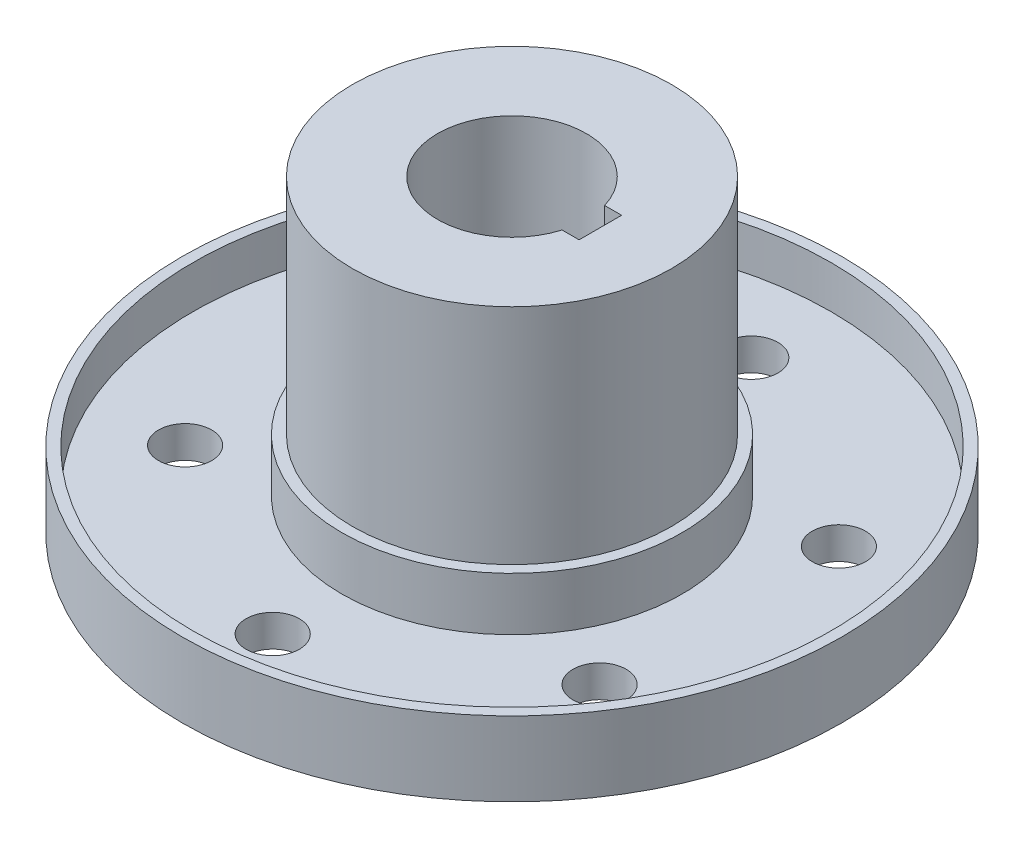
ISO-10303-21;
HEADER;
FILE_DESCRIPTION(('STEP AP214'),'2;1');
FILE_NAME('part.step','',(''),(''),'','','');
FILE_SCHEMA(('AUTOMOTIVE_DESIGN { 1 0 10303 214 1 1 1 1 }'));
ENDSEC;
DATA;
#1=APPLICATION_CONTEXT('core data for automotive mechanical design processes');
#2=APPLICATION_PROTOCOL_DEFINITION('international standard','automotive_design',2000,#1);
#3=PRODUCT_CONTEXT('',#1,'mechanical');
#4=PRODUCT('Part','Part','',(#3));
#5=PRODUCT_RELATED_PRODUCT_CATEGORY('part','',(#4));
#6=PRODUCT_DEFINITION_FORMATION('','',#4);
#7=PRODUCT_DEFINITION_CONTEXT('part definition',#1,'design');
#8=PRODUCT_DEFINITION('design','',#6,#7);
#9=PRODUCT_DEFINITION_SHAPE('','',#8);
#10=(LENGTH_UNIT() NAMED_UNIT(*) SI_UNIT(.MILLI.,.METRE.));
#11=(NAMED_UNIT(*) PLANE_ANGLE_UNIT() SI_UNIT($,.RADIAN.));
#12=(NAMED_UNIT(*) SI_UNIT($,.STERADIAN.) SOLID_ANGLE_UNIT());
#13=UNCERTAINTY_MEASURE_WITH_UNIT(LENGTH_MEASURE(1.E-05),#10,'distance_accuracy_value','');
#14=(GEOMETRIC_REPRESENTATION_CONTEXT(3) GLOBAL_UNCERTAINTY_ASSIGNED_CONTEXT((#13)) GLOBAL_UNIT_ASSIGNED_CONTEXT((#10,
#11,#12)) REPRESENTATION_CONTEXT('',''));
#15=CARTESIAN_POINT('',(0.,0.,0.));
#16=DIRECTION('',(0.,0.,1.));
#17=DIRECTION('',(1.,0.,0.));
#18=AXIS2_PLACEMENT_3D('',#15,#16,#17);
#19=CARTESIAN_POINT('',(41.5410196624969,2.99999999999998,-10.));
#20=DIRECTION('',(1.,0.,0.));
#21=DIRECTION('',(0.,0.,-1.));
#22=AXIS2_PLACEMENT_3D('',#19,#20,#21);
#23=PLANE('',#22);
#24=DIRECTION('',(0.,0.,-1.));
#25=VECTOR('',#24,1.);
#26=CARTESIAN_POINT('',(41.5410196624969,50.,-10.));
#27=LINE('',#26,#25);
#28=CARTESIAN_POINT('',(41.5410196624969,50.,9.99999999999999));
#29=VERTEX_POINT('',#28);
#30=CARTESIAN_POINT('',(41.5410196624969,50.,-10.));
#31=VERTEX_POINT('',#30);
#32=EDGE_CURVE('E52',#29,#31,#27,.T.);
#33=ORIENTED_EDGE('',*,*,#32,.F.);
#34=DIRECTION('',(0.,1.,0.));
#35=VECTOR('',#34,1.);
#36=CARTESIAN_POINT('',(41.5410196624969,2.99999999999998,9.99999999999999));
#37=LINE('',#36,#35);
#38=CARTESIAN_POINT('',(41.5410196624969,145.,9.99999999999999));
#39=VERTEX_POINT('',#38);
#40=EDGE_CURVE('E98',#29,#39,#37,.T.);
#41=ORIENTED_EDGE('',*,*,#40,.T.);
#42=DIRECTION('',(0.,0.,-1.));
#43=VECTOR('',#42,1.);
#44=CARTESIAN_POINT('',(41.5410196624969,145.,-10.));
#45=LINE('',#44,#43);
#46=CARTESIAN_POINT('',(41.5410196624969,145.,-10.));
#47=VERTEX_POINT('',#46);
#48=EDGE_CURVE('E372',#39,#47,#45,.T.);
#49=ORIENTED_EDGE('',*,*,#48,.T.);
#50=DIRECTION('',(0.,1.,0.));
#51=VECTOR('',#50,1.);
#52=CARTESIAN_POINT('',(41.5410196624969,2.99999999999998,-10.));
#53=LINE('',#52,#51);
#54=EDGE_CURVE('E58',#31,#47,#53,.T.);
#55=ORIENTED_EDGE('',*,*,#54,.F.);
#56=EDGE_LOOP('',(#33,#41,#49,#55));
#57=FACE_BOUND('',#56,.T.);
#58=ADVANCED_FACE('F39',(#57),#23,.F.);
#59=CARTESIAN_POINT('',(41.5410196624969,2.99999999999998,9.99999999999999));
#60=DIRECTION('',(0.,0.,1.));
#61=DIRECTION('',(1.,0.,0.));
#62=AXIS2_PLACEMENT_3D('',#59,#60,#61);
#63=PLANE('',#62);
#64=DIRECTION('',(1.,0.,0.));
#65=VECTOR('',#64,1.);
#66=CARTESIAN_POINT('',(41.5410196624969,50.,9.99999999999999));
#67=LINE('',#66,#65);
#68=CARTESIAN_POINT('',(33.5410196624969,50.,9.99999999999998));
#69=VERTEX_POINT('',#68);
#70=EDGE_CURVE('E88',#69,#29,#67,.T.);
#71=ORIENTED_EDGE('',*,*,#70,.F.);
#72=DIRECTION('',(0.,1.,0.));
#73=VECTOR('',#72,1.);
#74=CARTESIAN_POINT('',(33.5410196624969,2.99999999999998,9.99999999999998));
#75=LINE('',#74,#73);
#76=CARTESIAN_POINT('',(33.5410196624969,145.,9.99999999999998));
#77=VERTEX_POINT('',#76);
#78=EDGE_CURVE('E90',#69,#77,#75,.T.);
#79=ORIENTED_EDGE('',*,*,#78,.T.);
#80=DIRECTION('',(1.,0.,0.));
#81=VECTOR('',#80,1.);
#82=CARTESIAN_POINT('',(41.5410196624969,145.,9.99999999999999));
#83=LINE('',#82,#81);
#84=EDGE_CURVE('E96',#77,#39,#83,.T.);
#85=ORIENTED_EDGE('',*,*,#84,.T.);
#86=ORIENTED_EDGE('',*,*,#40,.F.);
#87=EDGE_LOOP('',(#71,#79,#85,#86));
#88=FACE_BOUND('',#87,.T.);
#89=ADVANCED_FACE('F185',(#88),#63,.F.);
#90=CARTESIAN_POINT('',(0.,2.99999999999998,0.));
#91=DIRECTION('',(0.,1.,0.));
#92=DIRECTION('',(0.,0.,1.));
#93=AXIS2_PLACEMENT_3D('',#90,#91,#92);
#94=CYLINDRICAL_SURFACE('',#93,35.);
#95=CARTESIAN_POINT('',(0.,50.,0.));
#96=DIRECTION('',(0.,-1.,0.));
#97=DIRECTION('',(0.,0.,-1.));
#98=AXIS2_PLACEMENT_3D('',#95,#96,#97);
#99=CIRCLE('',#98,35.);
#100=CARTESIAN_POINT('',(33.5410196624969,50.,-10.));
#101=VERTEX_POINT('',#100);
#102=EDGE_CURVE('E79',#101,#69,#99,.F.);
#103=ORIENTED_EDGE('',*,*,#102,.F.);
#104=DIRECTION('',(0.,1.,0.));
#105=VECTOR('',#104,1.);
#106=CARTESIAN_POINT('',(33.5410196624969,2.99999999999998,-10.));
#107=LINE('',#106,#105);
#108=CARTESIAN_POINT('',(33.5410196624969,145.,-10.));
#109=VERTEX_POINT('',#108);
#110=EDGE_CURVE('E86',#101,#109,#107,.T.);
#111=ORIENTED_EDGE('',*,*,#110,.T.);
#112=CARTESIAN_POINT('',(0.,145.,0.));
#113=DIRECTION('',(0.,1.,0.));
#114=DIRECTION('',(0.,0.,1.));
#115=AXIS2_PLACEMENT_3D('',#112,#113,#114);
#116=CIRCLE('',#115,35.);
#117=EDGE_CURVE('E380',#109,#77,#116,.T.);
#118=ORIENTED_EDGE('',*,*,#117,.T.);
#119=ORIENTED_EDGE('',*,*,#78,.F.);
#120=EDGE_LOOP('',(#103,#111,#118,#119));
#121=FACE_BOUND('',#120,.T.);
#122=ADVANCED_FACE('F81',(#121),#94,.F.);
#123=CARTESIAN_POINT('',(41.5410196624969,2.99999999999998,-10.));
#124=DIRECTION('',(0.,0.,-1.));
#125=DIRECTION('',(-1.,0.,0.));
#126=AXIS2_PLACEMENT_3D('',#123,#124,#125);
#127=PLANE('',#126);
#128=DIRECTION('',(-1.,0.,0.));
#129=VECTOR('',#128,1.);
#130=CARTESIAN_POINT('',(41.5410196624969,50.,-10.));
#131=LINE('',#130,#129);
#132=EDGE_CURVE('E11',#31,#101,#131,.T.);
#133=ORIENTED_EDGE('',*,*,#132,.F.);
#134=ORIENTED_EDGE('',*,*,#54,.T.);
#135=DIRECTION('',(-1.,0.,0.));
#136=VECTOR('',#135,1.);
#137=CARTESIAN_POINT('',(41.5410196624969,145.,-10.));
#138=LINE('',#137,#136);
#139=EDGE_CURVE('E92',#47,#109,#138,.T.);
#140=ORIENTED_EDGE('',*,*,#139,.T.);
#141=ORIENTED_EDGE('',*,*,#110,.F.);
#142=EDGE_LOOP('',(#133,#134,#140,#141));
#143=FACE_BOUND('',#142,.T.);
#144=ADVANCED_FACE('F91',(#143),#127,.F.);
#145=CARTESIAN_POINT('',(0.,35.,0.));
#146=DIRECTION('',(0.,1.,0.));
#147=DIRECTION('',(0.,0.,1.));
#148=AXIS2_PLACEMENT_3D('',#145,#146,#147);
#149=PLANE('',#148);
#150=CARTESIAN_POINT('',(0.,35.,0.));
#151=DIRECTION('',(0.,1.,0.));
#152=DIRECTION('',(0.,0.,1.));
#153=AXIS2_PLACEMENT_3D('',#150,#151,#152);
#154=CIRCLE('',#153,155.);
#155=CARTESIAN_POINT('',(0.,35.,155.));
#156=VERTEX_POINT('',#155);
#157=EDGE_CURVE('E152',#156,#156,#154,.T.);
#158=ORIENTED_EDGE('',*,*,#157,.T.);
#159=EDGE_LOOP('',(#158));
#160=FACE_BOUND('',#159,.T.);
#161=CARTESIAN_POINT('',(0.,35.,0.));
#162=DIRECTION('',(0.,1.,0.));
#163=DIRECTION('',(0.,0.,1.));
#164=AXIS2_PLACEMENT_3D('',#161,#162,#163);
#165=CIRCLE('',#164,150.);
#166=CARTESIAN_POINT('',(0.,35.,150.));
#167=VERTEX_POINT('',#166);
#168=EDGE_CURVE('E148',#167,#167,#165,.T.);
#169=ORIENTED_EDGE('',*,*,#168,.F.);
#170=EDGE_LOOP('',(#169));
#171=FACE_BOUND('',#170,.T.);
#172=ADVANCED_FACE('F169',(#160,#171),#149,.T.);
#173=CARTESIAN_POINT('',(0.,0.,0.));
#174=DIRECTION('',(0.,1.,0.));
#175=DIRECTION('',(0.,0.,1.));
#176=AXIS2_PLACEMENT_3D('',#173,#174,#175);
#177=PLANE('',#176);
#178=CARTESIAN_POINT('',(0.,0.,0.));
#179=DIRECTION('',(0.,-1.,0.));
#180=DIRECTION('',(0.,0.,-1.));
#181=AXIS2_PLACEMENT_3D('',#178,#179,#180);
#182=CIRCLE('',#181,60.);
#183=CARTESIAN_POINT('',(0.,0.,-60.));
#184=VERTEX_POINT('',#183);
#185=EDGE_CURVE('E368',#184,#184,#182,.T.);
#186=ORIENTED_EDGE('',*,*,#185,.F.);
#187=EDGE_LOOP('',(#186));
#188=FACE_BOUND('',#187,.T.);
#189=CARTESIAN_POINT('',(0.,0.,-112.5));
#190=DIRECTION('',(0.,1.,0.));
#191=DIRECTION('',(0.,0.,1.));
#192=AXIS2_PLACEMENT_3D('',#189,#190,#191);
#193=CIRCLE('',#192,12.5);
#194=CARTESIAN_POINT('',(0.,0.,-100.));
#195=VERTEX_POINT('',#194);
#196=EDGE_CURVE('E150',#195,#195,#193,.T.);
#197=ORIENTED_EDGE('',*,*,#196,.T.);
#198=EDGE_LOOP('',(#197));
#199=FACE_BOUND('',#198,.T.);
#200=CARTESIAN_POINT('',(-97.4278579257487,0.,-56.2500000000002));
#201=DIRECTION('',(0.,1.,0.));
#202=DIRECTION('',(0.,0.,1.));
#203=AXIS2_PLACEMENT_3D('',#200,#201,#202);
#204=CIRCLE('',#203,12.500000000001);
#205=CARTESIAN_POINT('',(-97.4278579257487,0.,-43.7499999999992));
#206=VERTEX_POINT('',#205);
#207=EDGE_CURVE('E144',#206,#206,#204,.T.);
#208=ORIENTED_EDGE('',*,*,#207,.T.);
#209=EDGE_LOOP('',(#208));
#210=FACE_BOUND('',#209,.T.);
#211=CARTESIAN_POINT('',(-97.4278579257485,0.,56.249999999999));
#212=DIRECTION('',(0.,1.,0.));
#213=DIRECTION('',(0.,0.,1.));
#214=AXIS2_PLACEMENT_3D('',#211,#212,#213);
#215=CIRCLE('',#214,12.5000000000009);
#216=CARTESIAN_POINT('',(-97.4278579257485,0.,68.75));
#217=VERTEX_POINT('',#216);
#218=EDGE_CURVE('E142',#217,#217,#215,.T.);
#219=ORIENTED_EDGE('',*,*,#218,.T.);
#220=EDGE_LOOP('',(#219));
#221=FACE_BOUND('',#220,.T.);
#222=CARTESIAN_POINT('',(2.51087448004034E-13,0.,112.499999999999));
#223=DIRECTION('',(0.,1.,0.));
#224=DIRECTION('',(0.,0.,1.));
#225=AXIS2_PLACEMENT_3D('',#222,#223,#224);
#226=CIRCLE('',#225,12.5000000000014);
#227=CARTESIAN_POINT('',(2.51087448004034E-13,0.,125.));
#228=VERTEX_POINT('',#227);
#229=EDGE_CURVE('E137',#228,#228,#226,.T.);
#230=ORIENTED_EDGE('',*,*,#229,.T.);
#231=EDGE_LOOP('',(#230));
#232=FACE_BOUND('',#231,.T.);
#233=CARTESIAN_POINT('',(97.4278579257489,0.,56.2499999999988));
#234=DIRECTION('',(0.,1.,0.));
#235=DIRECTION('',(0.,0.,1.));
#236=AXIS2_PLACEMENT_3D('',#233,#234,#235);
#237=CIRCLE('',#236,12.5000000000016);
#238=CARTESIAN_POINT('',(97.4278579257489,0.,68.7500000000004));
#239=VERTEX_POINT('',#238);
#240=EDGE_CURVE('E134',#239,#239,#237,.T.);
#241=ORIENTED_EDGE('',*,*,#240,.T.);
#242=EDGE_LOOP('',(#241));
#243=FACE_BOUND('',#242,.T.);
#244=CARTESIAN_POINT('',(97.4278579257488,0.,-56.2500000000005));
#245=DIRECTION('',(0.,1.,0.));
#246=DIRECTION('',(0.,0.,1.));
#247=AXIS2_PLACEMENT_3D('',#244,#245,#246);
#248=CIRCLE('',#247,12.500000000001);
#249=CARTESIAN_POINT('',(97.4278579257488,0.,-43.7499999999995));
#250=VERTEX_POINT('',#249);
#251=EDGE_CURVE('E117',#250,#250,#248,.T.);
#252=ORIENTED_EDGE('',*,*,#251,.T.);
#253=EDGE_LOOP('',(#252));
#254=FACE_BOUND('',#253,.T.);
#255=CARTESIAN_POINT('',(0.,0.,0.));
#256=DIRECTION('',(0.,1.,0.));
#257=DIRECTION('',(0.,0.,1.));
#258=AXIS2_PLACEMENT_3D('',#255,#256,#257);
#259=CIRCLE('',#258,155.);
#260=CARTESIAN_POINT('',(0.,0.,155.));
#261=VERTEX_POINT('',#260);
#262=EDGE_CURVE('E153',#261,#261,#259,.T.);
#263=ORIENTED_EDGE('',*,*,#262,.F.);
#264=EDGE_LOOP('',(#263));
#265=FACE_BOUND('',#264,.T.);
#266=ADVANCED_FACE('F171',(#188,#199,#210,#221,#232,#243,#254,#265),#177,.F.);
#267=CARTESIAN_POINT('',(0.,35.,0.));
#268=DIRECTION('',(0.,-1.,0.));
#269=DIRECTION('',(0.,0.,-1.));
#270=AXIS2_PLACEMENT_3D('',#267,#268,#269);
#271=CYLINDRICAL_SURFACE('',#270,155.);
#272=ORIENTED_EDGE('',*,*,#157,.F.);
#273=EDGE_LOOP('',(#272));
#274=FACE_BOUND('',#273,.T.);
#275=ORIENTED_EDGE('',*,*,#262,.T.);
#276=EDGE_LOOP('',(#275));
#277=FACE_BOUND('',#276,.T.);
#278=ADVANCED_FACE('F41',(#274,#277),#271,.T.);
#279=CARTESIAN_POINT('',(0.,35.,0.));
#280=DIRECTION('',(0.,-1.,0.));
#281=DIRECTION('',(0.,0.,-1.));
#282=AXIS2_PLACEMENT_3D('',#279,#280,#281);
#283=CYLINDRICAL_SURFACE('',#282,150.);
#284=CARTESIAN_POINT('',(0.,15.,0.));
#285=DIRECTION('',(0.,1.,0.));
#286=DIRECTION('',(0.,0.,1.));
#287=AXIS2_PLACEMENT_3D('',#284,#285,#286);
#288=CIRCLE('',#287,150.);
#289=CARTESIAN_POINT('',(0.,15.,150.));
#290=VERTEX_POINT('',#289);
#291=EDGE_CURVE('E108',#290,#290,#288,.T.);
#292=ORIENTED_EDGE('',*,*,#291,.F.);
#293=EDGE_LOOP('',(#292));
#294=FACE_BOUND('',#293,.T.);
#295=ORIENTED_EDGE('',*,*,#168,.T.);
#296=EDGE_LOOP('',(#295));
#297=FACE_BOUND('',#296,.T.);
#298=ADVANCED_FACE('F161',(#294,#297),#283,.F.);
#299=CARTESIAN_POINT('',(0.,15.,0.));
#300=DIRECTION('',(0.,1.,0.));
#301=DIRECTION('',(0.,0.,1.));
#302=AXIS2_PLACEMENT_3D('',#299,#300,#301);
#303=PLANE('',#302);
#304=CARTESIAN_POINT('',(0.,15.,0.));
#305=DIRECTION('',(0.,1.,0.));
#306=DIRECTION('',(0.,0.,1.));
#307=AXIS2_PLACEMENT_3D('',#304,#305,#306);
#308=CIRCLE('',#307,80.);
#309=CARTESIAN_POINT('',(0.,15.,80.));
#310=VERTEX_POINT('',#309);
#311=EDGE_CURVE('E102',#310,#310,#308,.T.);
#312=ORIENTED_EDGE('',*,*,#311,.F.);
#313=EDGE_LOOP('',(#312));
#314=FACE_BOUND('',#313,.T.);
#315=CARTESIAN_POINT('',(0.,15.,-112.5));
#316=DIRECTION('',(0.,1.,0.));
#317=DIRECTION('',(0.,0.,1.));
#318=AXIS2_PLACEMENT_3D('',#315,#316,#317);
#319=CIRCLE('',#318,12.5);
#320=CARTESIAN_POINT('',(0.,15.,-100.));
#321=VERTEX_POINT('',#320);
#322=EDGE_CURVE('E114',#321,#321,#319,.T.);
#323=ORIENTED_EDGE('',*,*,#322,.F.);
#324=EDGE_LOOP('',(#323));
#325=FACE_BOUND('',#324,.T.);
#326=CARTESIAN_POINT('',(-97.4278579257487,15.,-56.2500000000002));
#327=DIRECTION('',(0.,1.,0.));
#328=DIRECTION('',(0.,0.,1.));
#329=AXIS2_PLACEMENT_3D('',#326,#327,#328);
#330=CIRCLE('',#329,12.500000000001);
#331=CARTESIAN_POINT('',(-97.4278579257487,15.,-43.7499999999992));
#332=VERTEX_POINT('',#331);
#333=EDGE_CURVE('E115',#332,#332,#330,.T.);
#334=ORIENTED_EDGE('',*,*,#333,.F.);
#335=EDGE_LOOP('',(#334));
#336=FACE_BOUND('',#335,.T.);
#337=CARTESIAN_POINT('',(-97.4278579257485,15.,56.249999999999));
#338=DIRECTION('',(0.,1.,0.));
#339=DIRECTION('',(0.,0.,1.));
#340=AXIS2_PLACEMENT_3D('',#337,#338,#339);
#341=CIRCLE('',#340,12.5000000000009);
#342=CARTESIAN_POINT('',(-97.4278579257485,15.,68.75));
#343=VERTEX_POINT('',#342);
#344=EDGE_CURVE('E125',#343,#343,#341,.T.);
#345=ORIENTED_EDGE('',*,*,#344,.F.);
#346=EDGE_LOOP('',(#345));
#347=FACE_BOUND('',#346,.T.);
#348=CARTESIAN_POINT('',(2.51087448004034E-13,15.,112.499999999999));
#349=DIRECTION('',(0.,1.,0.));
#350=DIRECTION('',(0.,0.,1.));
#351=AXIS2_PLACEMENT_3D('',#348,#349,#350);
#352=CIRCLE('',#351,12.5000000000014);
#353=CARTESIAN_POINT('',(2.51087448004034E-13,15.,125.));
#354=VERTEX_POINT('',#353);
#355=EDGE_CURVE('E129',#354,#354,#352,.T.);
#356=ORIENTED_EDGE('',*,*,#355,.F.);
#357=EDGE_LOOP('',(#356));
#358=FACE_BOUND('',#357,.T.);
#359=CARTESIAN_POINT('',(97.4278579257489,15.,56.2499999999988));
#360=DIRECTION('',(0.,1.,0.));
#361=DIRECTION('',(0.,0.,1.));
#362=AXIS2_PLACEMENT_3D('',#359,#360,#361);
#363=CIRCLE('',#362,12.5000000000016);
#364=CARTESIAN_POINT('',(97.4278579257489,15.,68.7500000000004));
#365=VERTEX_POINT('',#364);
#366=EDGE_CURVE('E123',#365,#365,#363,.T.);
#367=ORIENTED_EDGE('',*,*,#366,.F.);
#368=EDGE_LOOP('',(#367));
#369=FACE_BOUND('',#368,.T.);
#370=CARTESIAN_POINT('',(97.4278579257488,15.,-56.2500000000005));
#371=DIRECTION('',(0.,1.,0.));
#372=DIRECTION('',(0.,0.,1.));
#373=AXIS2_PLACEMENT_3D('',#370,#371,#372);
#374=CIRCLE('',#373,12.500000000001);
#375=CARTESIAN_POINT('',(97.4278579257488,15.,-43.7499999999995));
#376=VERTEX_POINT('',#375);
#377=EDGE_CURVE('E118',#376,#376,#374,.T.);
#378=ORIENTED_EDGE('',*,*,#377,.F.);
#379=EDGE_LOOP('',(#378));
#380=FACE_BOUND('',#379,.T.);
#381=ORIENTED_EDGE('',*,*,#291,.T.);
#382=EDGE_LOOP('',(#381));
#383=FACE_BOUND('',#382,.T.);
#384=ADVANCED_FACE('F163',(#314,#325,#336,#347,#358,#369,#380,#383),#303,.T.);
#385=CARTESIAN_POINT('',(97.4278579257488,-50.,-56.2500000000005));
#386=DIRECTION('',(0.,1.,0.));
#387=DIRECTION('',(0.,0.,1.));
#388=AXIS2_PLACEMENT_3D('',#385,#386,#387);
#389=CYLINDRICAL_SURFACE('',#388,12.500000000001);
#390=ORIENTED_EDGE('',*,*,#377,.T.);
#391=EDGE_LOOP('',(#390));
#392=FACE_BOUND('',#391,.T.);
#393=ORIENTED_EDGE('',*,*,#251,.F.);
#394=EDGE_LOOP('',(#393));
#395=FACE_BOUND('',#394,.T.);
#396=ADVANCED_FACE('F220',(#392,#395),#389,.F.);
#397=CARTESIAN_POINT('',(97.4278579257489,-50.,56.2499999999988));
#398=DIRECTION('',(0.,1.,0.));
#399=DIRECTION('',(0.,0.,1.));
#400=AXIS2_PLACEMENT_3D('',#397,#398,#399);
#401=CYLINDRICAL_SURFACE('',#400,12.5000000000016);
#402=ORIENTED_EDGE('',*,*,#366,.T.);
#403=EDGE_LOOP('',(#402));
#404=FACE_BOUND('',#403,.T.);
#405=ORIENTED_EDGE('',*,*,#240,.F.);
#406=EDGE_LOOP('',(#405));
#407=FACE_BOUND('',#406,.T.);
#408=ADVANCED_FACE('F219',(#404,#407),#401,.F.);
#409=CARTESIAN_POINT('',(2.51087448004034E-13,-50.,112.499999999999));
#410=DIRECTION('',(0.,1.,0.));
#411=DIRECTION('',(0.,0.,1.));
#412=AXIS2_PLACEMENT_3D('',#409,#410,#411);
#413=CYLINDRICAL_SURFACE('',#412,12.5000000000014);
#414=ORIENTED_EDGE('',*,*,#355,.T.);
#415=EDGE_LOOP('',(#414));
#416=FACE_BOUND('',#415,.T.);
#417=ORIENTED_EDGE('',*,*,#229,.F.);
#418=EDGE_LOOP('',(#417));
#419=FACE_BOUND('',#418,.T.);
#420=ADVANCED_FACE('F223',(#416,#419),#413,.F.);
#421=CARTESIAN_POINT('',(-97.4278579257485,-50.,56.249999999999));
#422=DIRECTION('',(0.,1.,0.));
#423=DIRECTION('',(0.,0.,1.));
#424=AXIS2_PLACEMENT_3D('',#421,#422,#423);
#425=CYLINDRICAL_SURFACE('',#424,12.5000000000009);
#426=ORIENTED_EDGE('',*,*,#344,.T.);
#427=EDGE_LOOP('',(#426));
#428=FACE_BOUND('',#427,.T.);
#429=ORIENTED_EDGE('',*,*,#218,.F.);
#430=EDGE_LOOP('',(#429));
#431=FACE_BOUND('',#430,.T.);
#432=ADVANCED_FACE('F213',(#428,#431),#425,.F.);
#433=CARTESIAN_POINT('',(-97.4278579257487,-50.,-56.2500000000002));
#434=DIRECTION('',(0.,1.,0.));
#435=DIRECTION('',(0.,0.,1.));
#436=AXIS2_PLACEMENT_3D('',#433,#434,#435);
#437=CYLINDRICAL_SURFACE('',#436,12.500000000001);
#438=ORIENTED_EDGE('',*,*,#333,.T.);
#439=EDGE_LOOP('',(#438));
#440=FACE_BOUND('',#439,.T.);
#441=ORIENTED_EDGE('',*,*,#207,.F.);
#442=EDGE_LOOP('',(#441));
#443=FACE_BOUND('',#442,.T.);
#444=ADVANCED_FACE('F212',(#440,#443),#437,.F.);
#445=CARTESIAN_POINT('',(0.,-50.,-112.5));
#446=DIRECTION('',(0.,1.,0.));
#447=DIRECTION('',(0.,0.,1.));
#448=AXIS2_PLACEMENT_3D('',#445,#446,#447);
#449=CYLINDRICAL_SURFACE('',#448,12.5);
#450=ORIENTED_EDGE('',*,*,#322,.T.);
#451=EDGE_LOOP('',(#450));
#452=FACE_BOUND('',#451,.T.);
#453=ORIENTED_EDGE('',*,*,#196,.F.);
#454=EDGE_LOOP('',(#453));
#455=FACE_BOUND('',#454,.T.);
#456=ADVANCED_FACE('F210',(#452,#455),#449,.F.);
#457=CARTESIAN_POINT('',(0.,40.,0.));
#458=DIRECTION('',(0.,-1.,0.));
#459=DIRECTION('',(0.,0.,-1.));
#460=AXIS2_PLACEMENT_3D('',#457,#458,#459);
#461=CYLINDRICAL_SURFACE('',#460,80.);
#462=CARTESIAN_POINT('',(0.,40.,0.));
#463=DIRECTION('',(0.,1.,0.));
#464=DIRECTION('',(0.,0.,1.));
#465=AXIS2_PLACEMENT_3D('',#462,#463,#464);
#466=CIRCLE('',#465,80.);
#467=CARTESIAN_POINT('',(0.,40.,80.));
#468=VERTEX_POINT('',#467);
#469=EDGE_CURVE('E107',#468,#468,#466,.T.);
#470=ORIENTED_EDGE('',*,*,#469,.F.);
#471=EDGE_LOOP('',(#470));
#472=FACE_BOUND('',#471,.T.);
#473=ORIENTED_EDGE('',*,*,#311,.T.);
#474=EDGE_LOOP('',(#473));
#475=FACE_BOUND('',#474,.T.);
#476=ADVANCED_FACE('F202',(#472,#475),#461,.T.);
#477=CARTESIAN_POINT('',(0.,40.,0.));
#478=DIRECTION('',(0.,1.,0.));
#479=DIRECTION('',(0.,0.,1.));
#480=AXIS2_PLACEMENT_3D('',#477,#478,#479);
#481=PLANE('',#480);
#482=CARTESIAN_POINT('',(0.,40.,0.));
#483=DIRECTION('',(0.,1.,0.));
#484=DIRECTION('',(0.,0.,1.));
#485=AXIS2_PLACEMENT_3D('',#482,#483,#484);
#486=CIRCLE('',#485,75.);
#487=CARTESIAN_POINT('',(0.,40.,75.));
#488=VERTEX_POINT('',#487);
#489=EDGE_CURVE('E50',#488,#488,#486,.T.);
#490=ORIENTED_EDGE('',*,*,#489,.F.);
#491=EDGE_LOOP('',(#490));
#492=FACE_BOUND('',#491,.T.);
#493=ORIENTED_EDGE('',*,*,#469,.T.);
#494=EDGE_LOOP('',(#493));
#495=FACE_BOUND('',#494,.T.);
#496=ADVANCED_FACE('F197',(#492,#495),#481,.T.);
#497=CARTESIAN_POINT('',(0.,145.,0.));
#498=DIRECTION('',(0.,-1.,0.));
#499=DIRECTION('',(0.,0.,-1.));
#500=AXIS2_PLACEMENT_3D('',#497,#498,#499);
#501=CYLINDRICAL_SURFACE('',#500,75.);
#502=CARTESIAN_POINT('',(0.,145.,0.));
#503=DIRECTION('',(0.,1.,0.));
#504=DIRECTION('',(0.,0.,1.));
#505=AXIS2_PLACEMENT_3D('',#502,#503,#504);
#506=CIRCLE('',#505,75.);
#507=CARTESIAN_POINT('',(0.,145.,75.));
#508=VERTEX_POINT('',#507);
#509=EDGE_CURVE('E105',#508,#508,#506,.T.);
#510=ORIENTED_EDGE('',*,*,#509,.F.);
#511=EDGE_LOOP('',(#510));
#512=FACE_BOUND('',#511,.T.);
#513=ORIENTED_EDGE('',*,*,#489,.T.);
#514=EDGE_LOOP('',(#513));
#515=FACE_BOUND('',#514,.T.);
#516=ADVANCED_FACE('F193',(#512,#515),#501,.T.);
#517=CARTESIAN_POINT('',(0.,145.,0.));
#518=DIRECTION('',(0.,1.,0.));
#519=DIRECTION('',(0.,0.,1.));
#520=AXIS2_PLACEMENT_3D('',#517,#518,#519);
#521=PLANE('',#520);
#522=ORIENTED_EDGE('',*,*,#48,.F.);
#523=ORIENTED_EDGE('',*,*,#84,.F.);
#524=ORIENTED_EDGE('',*,*,#117,.F.);
#525=ORIENTED_EDGE('',*,*,#139,.F.);
#526=EDGE_LOOP('',(#522,#523,#524,#525));
#527=FACE_BOUND('',#526,.T.);
#528=ORIENTED_EDGE('',*,*,#509,.T.);
#529=EDGE_LOOP('',(#528));
#530=FACE_BOUND('',#529,.T.);
#531=ADVANCED_FACE('F194',(#527,#530),#521,.T.);
#532=CARTESIAN_POINT('',(0.,50.,0.));
#533=DIRECTION('',(0.,-1.,0.));
#534=DIRECTION('',(0.,0.,-1.));
#535=AXIS2_PLACEMENT_3D('',#532,#533,#534);
#536=PLANE('',#535);
#537=CARTESIAN_POINT('',(0.,50.,0.));
#538=DIRECTION('',(0.,-1.,0.));
#539=DIRECTION('',(0.,0.,-1.));
#540=AXIS2_PLACEMENT_3D('',#537,#538,#539);
#541=CIRCLE('',#540,60.);
#542=CARTESIAN_POINT('',(0.,50.,-60.));
#543=VERTEX_POINT('',#542);
#544=EDGE_CURVE('E87',#543,#543,#541,.T.);
#545=ORIENTED_EDGE('',*,*,#544,.T.);
#546=EDGE_LOOP('',(#545));
#547=FACE_BOUND('',#546,.T.);
#548=ORIENTED_EDGE('',*,*,#32,.T.);
#549=ORIENTED_EDGE('',*,*,#132,.T.);
#550=ORIENTED_EDGE('',*,*,#102,.T.);
#551=ORIENTED_EDGE('',*,*,#70,.T.);
#552=EDGE_LOOP('',(#548,#549,#550,#551));
#553=FACE_BOUND('',#552,.T.);
#554=ADVANCED_FACE('F76',(#547,#553),#536,.T.);
#555=CARTESIAN_POINT('',(0.,50.,0.));
#556=DIRECTION('',(0.,-1.,0.));
#557=DIRECTION('',(0.,0.,-1.));
#558=AXIS2_PLACEMENT_3D('',#555,#556,#557);
#559=CYLINDRICAL_SURFACE('',#558,60.);
#560=ORIENTED_EDGE('',*,*,#544,.F.);
#561=EDGE_LOOP('',(#560));
#562=FACE_BOUND('',#561,.T.);
#563=ORIENTED_EDGE('',*,*,#185,.T.);
#564=EDGE_LOOP('',(#563));
#565=FACE_BOUND('',#564,.T.);
#566=ADVANCED_FACE('F349',(#562,#565),#559,.F.);
#567=CLOSED_SHELL('',(#58,#89,#122,#144,#172,#266,#278,#298,#384,#396,#408,#420,#432,#444,#456,
#476,#496,#516,#531,#554,#566));
#568=MANIFOLD_SOLID_BREP('B2',#567);
#569=ADVANCED_BREP_SHAPE_REPRESENTATION('',(#18,#568),#14);
#570=SHAPE_DEFINITION_REPRESENTATION(#9,#569);
ENDSEC;
END-ISO-10303-21;
